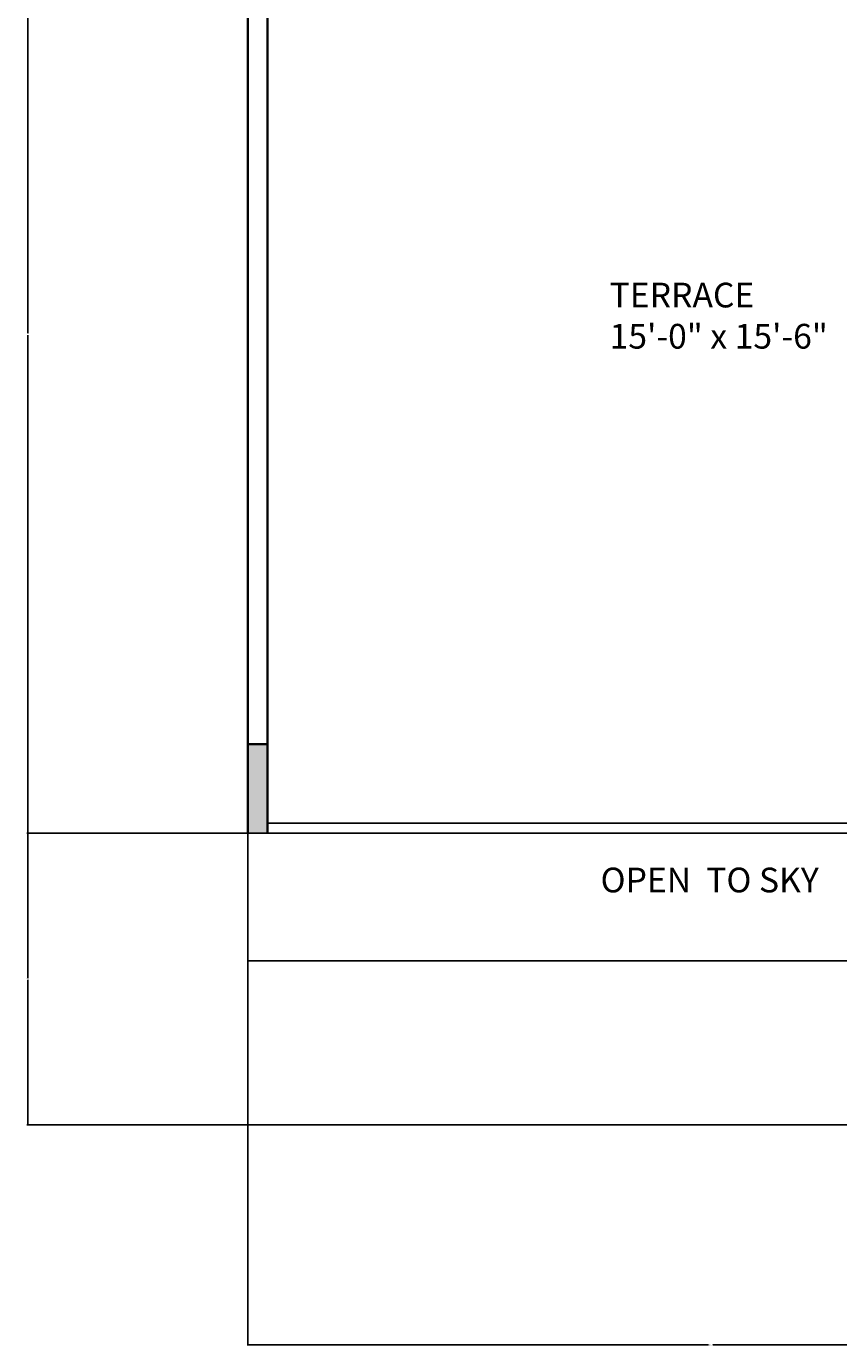
# Model space of a CAD drawing. Units: inches. Extents: x 1002 to 1561, y 1016 to 1994.
# Tile 1 of 8: x 1002 to 1166, y 1016 to 1283. Entities that reach past the tile are written whole.
import ezdxf

# ---------------------------------------------------------------- set-up
doc = ezdxf.new("R2010")
doc.units = ezdxf.units.IN
doc.header["$MEASUREMENT"] = 0
for name, color, linetype, lineweight in [('A-ANNO-DIMS', 2, 'Continuous', 18), ('A-AREA-IDEN', 7, 'Continuous', 18), ('A-WALL', 7, 'Continuous', 35), ('A-WALL-PATT', 7, 'Continuous', 13)]:
    doc.layers.add(name, color=color, linetype=linetype, lineweight=lineweight)
doc.layers.add('A-FLOR-EDGE', color=217, linetype='Continuous', lineweight=25, true_color=0x93278f)
doc.styles.get("Standard").update_dxf_attribs({"font": 'arial.ttf'})
doc.dimstyles.get("Standard").update_dxf_attribs({"dimtxt": 0.18, "dimasz": 0.18, "dimexe": 0.18, "dimexo": 0.0625, "dimgap": 0.09, "dimtad": 0, "dimtih": 1, "dimtoh": 1, "dimdec": 4, "dimzin": 0, "dimdsep": 46, "dimtxsty": 'Standard', "dimcen": 0.09, "dimadec": 0, "dimazin": 0, "dimtfac": 1, "dimtdec": 4, "dimtofl": 0, "dimtmove": 0, "dimatfit": 3, "dimfxl": 1, "dimtolj": 1, "dimtzin": 0, "dimarcsym": 0})

# ---------------------------------------------------------------- blocks, each defined once
blk = doc.blocks.new('*D15')
at = {"layer": 'A-ANNO-DIMS', "color": 0, "lineweight": -2, "transparency": 16777216}
for p, q in [((1046.37, 1321.51), (1001.74, 1321.51)), ((1001.92, 1321.33), (1001.92, 1220.69)), ((1001.92, 1119.69), (1001.92, 1220.33)), ((1046.37, 1119.51), (1001.74, 1119.51))]:
    blk.add_line(p, q, dxfattribs=at)
at = {"layer": 'A-ANNO-DIMS', "color": 0, "transparency": 16777216}
for points in [[(1001.89, 1321.33), (1001.95, 1321.33), (1001.92, 1321.51)], [(1001.89, 1119.69), (1001.95, 1119.69), (1001.92, 1119.51)]]:
    blk.add_solid(points, dxfattribs=at)
at = {"layer": 'Defpoints', "color": 0, "transparency": 16777216}
for p in [(1001.92, 1321.51), (1046.43, 1321.51), (1046.43, 1119.51)]:
    blk.add_point(p, dxfattribs=at)
at = {"layer": 'A-ANNO-DIMS', "color": 0, "transparency": 16777216, "insert": (1001.92, 1220.51), "char_height": 0.18, "attachment_point": 5}
blk.add_mtext('\\A1;202', dxfattribs=at)
blk = doc.blocks.new('*D16')
at = {"layer": 'A-ANNO-DIMS', "color": 0, "lineweight": -2, "transparency": 16777216}
for p, q in [((1046.37, 1119.51), (1001.74, 1119.51)), ((1001.92, 1119.33), (1001.92, 1090.18)), ((1001.92, 1060.67), (1001.92, 1089.82)), ((1281.73, 1060.49), (1001.74, 1060.49))]:
    blk.add_line(p, q, dxfattribs=at)
at = {"layer": 'A-ANNO-DIMS', "color": 0, "transparency": 16777216}
for points in [[(1001.89, 1119.33), (1001.95, 1119.33), (1001.92, 1119.51)], [(1001.89, 1060.67), (1001.95, 1060.67), (1001.92, 1060.49)]]:
    blk.add_solid(points, dxfattribs=at)
at = {"layer": 'Defpoints', "color": 0, "transparency": 16777216}
for p in [(1001.92, 1119.51), (1046.43, 1119.51), (1281.79, 1060.49)]:
    blk.add_point(p, dxfattribs=at)
at = {"layer": 'A-ANNO-DIMS', "color": 0, "transparency": 16777216, "insert": (1001.92, 1090), "char_height": 0.18, "attachment_point": 5}
blk.add_mtext('\\A1;59.02', dxfattribs=at)
blk = doc.blocks.new('*D17')
at = {"layer": 'A-ANNO-DIMS', "color": 0, "lineweight": -2, "transparency": 16777216}
for p, q in [((1233.77, 1119.45), (1233.77, 1015.8)), ((1046.43, 1093.59), (1046.43, 1015.8)), ((1046.61, 1015.98), (1139.65, 1015.98)), ((1233.59, 1015.98), (1140.56, 1015.98))]:
    blk.add_line(p, q, dxfattribs=at)
at = {"layer": 'A-ANNO-DIMS', "color": 0, "transparency": 16777216}
for points in [[(1046.61, 1016.01), (1046.61, 1015.95), (1046.43, 1015.98)], [(1233.59, 1016.01), (1233.59, 1015.95), (1233.77, 1015.98)]]:
    blk.add_solid(points, dxfattribs=at)
at = {"layer": 'Defpoints', "color": 0, "transparency": 16777216}
for p in [(1233.77, 1119.51), (1046.43, 1093.65), (1233.77, 1015.98)]:
    blk.add_point(p, dxfattribs=at)
at = {"layer": 'A-ANNO-DIMS', "color": 0, "transparency": 16777216, "insert": (1140.1, 1015.98), "char_height": 0.18, "attachment_point": 5}
blk.add_mtext('\\A1;187.34', dxfattribs=at)

msp = doc.modelspace()

# ---------------------------------------------------------------- hatches: boundary and pattern name
at = {"layer": 'A-WALL-PATT'}
h = msp.add_hatch(color=256, dxfattribs=at)
h.dxf.hatch_style = 1
h.paths.add_polyline_path([(1206.434, 1924.784), (1203.434, 1924.784), (1203.434, 1898.155), (1206.434, 1898.155)])
h.paths.add_polyline_path([(1326.434, 1925.745), (1323.434, 1925.745), (1323.434, 1900.458), (1326.434, 1900.458)])
h.paths.add_polyline_path([(1290.434, 1840.51), (1287.434, 1840.51), (1287.434, 1837.51), (1287.434, 1823.284), (1290.434, 1823.284)])
h.paths.add_polyline_path([(1287.434, 1840.51), (1285.684, 1840.51), (1285.684, 1837.51), (1287.434, 1837.51)])
h.paths.add_polyline_path([(1233.434, 1840.51), (1230.434, 1840.51), (1230.434, 1823.284), (1233.434, 1823.284)])
h.paths.add_polyline_path([(1235.119, 1840.51), (1233.434, 1840.51), (1233.434, 1837.51), (1235.119, 1837.51)])
h.paths.add_polyline_path([(1050.434, 1837.51), (1050.434, 1840.51), (1046.434, 1840.51), (1046.434, 1814.619), (1050.434, 1814.619)])
h.paths.add_polyline_path([(1050.434, 1682.088), (1046.434, 1682.088), (1046.434, 1648.51), (1046.434, 1645.51), (1050.434, 1645.51), (1050.434, 1648.51)])
h.paths.add_polyline_path([(1233.434, 1648.51), (1211.636, 1648.51), (1211.636, 1645.51), (1233.434, 1645.51)])
h.paths.add_polyline_path([(1307.549, 1648.51), (1287.434, 1648.51), (1287.434, 1645.51), (1307.549, 1645.51)])
h.paths.add_polyline_path([(1516.434, 1927.595), (1512.434, 1927.595), (1512.434, 1896.846), (1516.434, 1896.846)])
h.paths.add_polyline_path([(1516.434, 1840.51), (1512.434, 1840.51), (1512.434, 1816.31), (1516.434, 1816.31)])
h.paths.add_polyline_path([(1516.434, 1686.827), (1512.434, 1686.827), (1512.434, 1645.51), (1516.434, 1645.51)])
h.paths.add_polyline_path([(1472.434, 1321.51), (1469.434, 1321.51), (1469.434, 1306.51), (1472.434, 1306.51)])
h.paths.add_polyline_path([(1295.733, 1141.51), (1281.793, 1141.51), (1281.793, 1137.51), (1295.733, 1137.51)])
h.paths.add_polyline_path([(1239.434, 1321.51), (1230.434, 1321.51), (1230.434, 1318.51), (1239.434, 1318.51)])
h.paths.add_polyline_path([(1290.434, 1332.122), (1287.434, 1332.122), (1287.434, 1318.51), (1290.434, 1318.51)])
h.paths.add_polyline_path([(1311.434, 1480.51), (1287.434, 1480.51), (1287.434, 1477.51), (1311.434, 1477.51)])
h.paths.add_polyline_path([(1050.434, 1480.51), (1046.434, 1480.51), (1046.434, 1468.51), (1050.434, 1468.51)])
h.paths.add_polyline_path([(1050.434, 1321.51), (1046.434, 1321.51), (1046.434, 1309.51), (1050.434, 1309.51)])
h.paths.add_polyline_path([(1233.434, 1192.382), (1230.434, 1192.382), (1230.434, 1168.702), (1233.434, 1168.702)])
h.paths.add_polyline_path([(1050.434, 1137.51), (1046.434, 1137.51), (1046.434, 1119.51), (1050.434, 1119.51)])
h.paths.add_polyline_path([(1472.434, 1153.51), (1469.434, 1153.51), (1469.434, 1141.51), (1472.434, 1141.51)])
h.paths.add_polyline_path([(1472.434, 1141.51), (1469.434, 1141.51), (1469.434, 1137.51), (1472.434, 1137.51)])

# ---------------------------------------------------------------- linework, layer by layer
at = {"layer": 'A-FLOR-EDGE'}
for p, q in [((1050.434, 1121.51), (1230.434, 1121.51)), ((1046.434, 1119.51), (1233.773, 1119.51)), ((1046.434, 1119.51), (1046.434, 1093.652)), ((1281.793, 1093.652), (1046.434, 1093.652))]:
    msp.add_line(p, q, dxfattribs=at)
at = {"layer": 'A-WALL'}
for p, q in [((1046.434, 1119.51), (1046.434, 1682.088)), ((1050.434, 1119.51), (1050.434, 1682.088)), ((1050.434, 1137.51), (1046.434, 1137.51))]:
    msp.add_line(p, q, dxfattribs=at)

# ---------------------------------------------------------------- texts
at = {"layer": 'A-AREA-IDEN', "char_height": 5, "attachment_point": 1}
for s, insert in [('TERRACE\\P15\'-0" x 15\'-6"', (1119.652, 1230.929)), ('OPEN  TO SKY', (1117.82, 1112.54))]:
    msp.add_mtext_dynamic_manual_height_columns(s, width=50.5101, gutter_width=1, heights=[0], dxfattribs=dict(at, insert=insert))

# ---------------------------------------------------------------- dimensions: what is measured, and where the dimension line sits
at = {"layer": 'A-ANNO-DIMS'}
for base, p1, p2, override, picture, middle in [((1001.924, 1321.51), (1046.434, 1119.51), (1046.434, 1321.51), {"dimdec": 0, "dimlfac": 1, "dimrnd": 0, "dimzin": 0, "dimdsep": 46, "dimlunit": 2}, '*D15', (1001.924, 1220.51)), ((1001.924, 1119.51), (1281.793, 1060.49), (1046.434, 1119.51), {"dimdec": 2, "dimlfac": 1, "dimrnd": 0, "dimzin": 0, "dimdsep": 46, "dimlunit": 2}, '*D16', (1001.924, 1090))]:
    dim = msp.add_linear_dim(base=base, p1=p1, p2=p2, angle=90, dimstyle='Standard', override=override, dxfattribs=at)
    dim.commit()
    dim.dimension.update_dxf_attribs({"geometry": picture, "text_midpoint": middle})
dim = msp.add_linear_dim(base=(1233.773, 1015.98), p1=(1046.434, 1093.652), p2=(1233.773, 1119.51), dimstyle='Standard', override={"dimdec": 2, "dimlfac": 1, "dimrnd": 0, "dimzin": 0, "dimdsep": 46, "dimlunit": 2}, dxfattribs=at)
dim.commit()
dim.dimension.update_dxf_attribs({"geometry": '*D17', "text_midpoint": (1140.103, 1015.98)})

doc.saveas('drawing.dxf')
